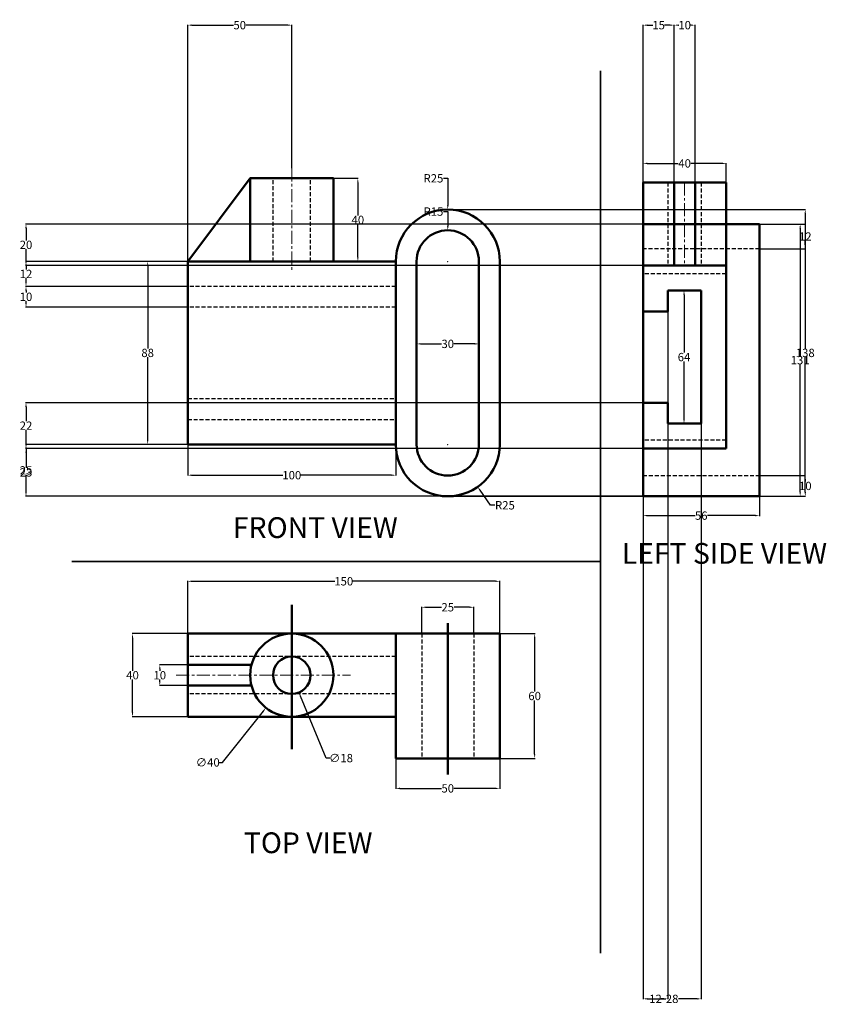
# Model space of a CAD drawing. Units: millimetres. Extents: x -141 to 252, y -566 to 219.
# Tile 1 of 2: x -141 to 247, y -566 to -92. Entities that reach past the tile are written whole.
import ezdxf

# ---------------------------------------------------------------- set-up
doc = ezdxf.new("R2010")
doc.units = ezdxf.units.MM
doc.header["$MEASUREMENT"] = 0
doc.linetypes.add('CENTER', pattern=[2, 1.25, -0.25, 0.25, -0.25])
doc.linetypes.add('HIDDEN', pattern=[9.525, 6.35, -3.175])
for name, color, linetype, lineweight in [('M-CNTR', 1, 'CENTER', 18), ('M-DIMS', 2, 'Continuous', 25), ('M-HIDN', 2, 'HIDDEN', 25), ('M-OUTL', 7, 'Continuous', 50), ('M-TEXT', 7, 'Continuous', 25), ('M-TTLB', 8, 'Continuous', 35)]:
    doc.layers.add(name, color=color, linetype=linetype, lineweight=lineweight)
doc.styles.get("Standard").update_dxf_attribs({"font": 'arial.ttf'})
doc.dimstyles.get("Standard").update_dxf_attribs({"dimtxt": 4, "dimasz": 2, "dimexe": 0.18, "dimexo": 0.0625, "dimgap": 0.09, "dimtad": 0, "dimtih": 1, "dimtoh": 1, "dimdec": 0, "dimzin": 0, "dimdsep": 46, "dimtxsty": 'Standard', "dimcen": 0.09, "dimadec": 0, "dimazin": 0, "dimtfac": 1, "dimtdec": 0, "dimtofl": 0, "dimtmove": 0, "dimatfit": 3, "dimfxl": 1, "dimtolj": 1, "dimtzin": 0, "dimarcsym": 0})

# ---------------------------------------------------------------- blocks, each defined once
blk = doc.blocks.new('*D12')
at = {"layer": 'Defpoints', "color": 0, "transparency": 16777216}
for p in [(-59.91, -208.36), (-79.17, -296.36), (-59.91, -296.36)]:
    blk.add_point(p, dxfattribs=at)
at = {"layer": 'M-DIMS', "color": 0, "lineweight": -2, "transparency": 16777216}
for p, q in [((-59.97, -208.36), (-79.35, -208.36)), ((-79.17, -210.36), (-79.17, -250.22)), ((-79.17, -294.36), (-79.17, -254.49)), ((-59.97, -296.36), (-79.35, -296.36))]:
    blk.add_line(p, q, dxfattribs=at)
at = {"layer": 'M-DIMS', "color": 0, "transparency": 16777216}
for points in [[(-79.5, -210.36), (-78.84, -210.36), (-79.17, -208.36)], [(-79.5, -294.36), (-78.84, -294.36), (-79.17, -296.36)]]:
    blk.add_solid(points, dxfattribs=at)
at = {"layer": 'M-DIMS', "color": 0, "transparency": 16777216, "insert": (-79.17, -252.36), "char_height": 4, "attachment_point": 5}
blk.add_mtext('\\A1;88', dxfattribs=at)
blk = doc.blocks.new('*D13')
at = {"layer": 'Defpoints', "color": 0, "transparency": 16777216}
for p in [(-59.91, -296.36), (40.09, -296.36), (40.09, -311.2)]:
    blk.add_point(p, dxfattribs=at)
at = {"layer": 'M-DIMS', "color": 0, "lineweight": -2, "transparency": 16777216}
for p, q in [((-59.91, -296.42), (-59.91, -311.38)), ((40.09, -296.42), (40.09, -311.38)), ((-57.91, -311.2), (-14.22, -311.2)), ((38.09, -311.2), (-5.59, -311.2))]:
    blk.add_line(p, q, dxfattribs=at)
at = {"layer": 'M-DIMS', "color": 0, "transparency": 16777216}
for points in [[(-57.91, -310.87), (-57.91, -311.54), (-59.91, -311.2)], [(38.09, -310.87), (38.09, -311.54), (40.09, -311.2)]]:
    blk.add_solid(points, dxfattribs=at)
at = {"layer": 'M-DIMS', "color": 0, "transparency": 16777216, "insert": (-9.91, -311.2), "char_height": 4, "attachment_point": 5}
blk.add_mtext('\\A1;100', dxfattribs=at)
blk = doc.blocks.new('*D14')
at = {"layer": 'Defpoints', "color": 0, "transparency": 16777216}
for p in [(10.09, -168.36), (21.87, -168.36), (10.09, -208.36)]:
    blk.add_point(p, dxfattribs=at)
at = {"layer": 'M-DIMS', "color": 0, "lineweight": -2, "transparency": 16777216}
for p, q in [((10.15, -168.36), (22.05, -168.36)), ((21.87, -170.36), (21.87, -186.22)), ((21.87, -206.36), (21.87, -190.49)), ((10.15, -208.36), (22.05, -208.36))]:
    blk.add_line(p, q, dxfattribs=at)
at = {"layer": 'M-DIMS', "color": 0, "transparency": 16777216}
for points in [[(21.54, -170.36), (22.2, -170.36), (21.87, -168.36)], [(21.54, -206.36), (22.2, -206.36), (21.87, -208.36)]]:
    blk.add_solid(points, dxfattribs=at)
at = {"layer": 'M-DIMS', "color": 0, "transparency": 16777216, "insert": (21.87, -188.36), "char_height": 4, "attachment_point": 5}
blk.add_mtext('\\A1;40', dxfattribs=at)
blk = doc.blocks.new('*D15')
at = {"layer": 'Defpoints', "color": 0, "transparency": 16777216}
for p in [(80.09, -248.02), (50.09, -252.36), (80.09, -252.36)]:
    blk.add_point(p, dxfattribs=at)
at = {"layer": 'M-DIMS', "color": 0, "lineweight": -2, "transparency": 16777216}
for p, q in [((50.09, -252.29), (50.09, -247.84)), ((52.09, -248.02), (62.15, -248.02)), ((78.09, -248.02), (68.04, -248.02)), ((80.09, -252.29), (80.09, -247.84))]:
    blk.add_line(p, q, dxfattribs=at)
at = {"layer": 'M-DIMS', "color": 0, "transparency": 16777216}
for points in [[(52.09, -247.69), (52.09, -248.36), (50.09, -248.02)], [(78.09, -247.69), (78.09, -248.36), (80.09, -248.02)]]:
    blk.add_solid(points, dxfattribs=at)
at = {"layer": 'M-DIMS', "color": 0, "transparency": 16777216, "insert": (65.09, -248.02), "char_height": 4, "attachment_point": 5}
blk.add_mtext('\\A1;30', dxfattribs=at)
blk = doc.blocks.new('*D16')
at = {"layer": 'Defpoints', "color": 0, "transparency": 16777216}
for p in [(65.09, -296.36), (79.46, -316.81)]:
    blk.add_point(p, dxfattribs=at)
at = {"layer": 'M-DIMS', "color": 0, "lineweight": -2, "transparency": 16777216}
for p, q in [((65, -296.36), (65.18, -296.36)), ((65.09, -296.45), (65.09, -296.27)), ((85.69, -325.67), (80.61, -318.45)), ((87.69, -325.67), (85.69, -325.67))]:
    blk.add_line(p, q, dxfattribs=at)
at = {"layer": 'M-DIMS', "color": 0, "transparency": 16777216}
blk.add_solid([(80.89, -318.26), (80.34, -318.64), (79.46, -316.81)], dxfattribs=at)
at = {"layer": 'M-DIMS', "color": 0, "transparency": 16777216, "insert": (92.57, -325.67), "char_height": 4, "attachment_point": 5}
blk.add_mtext('\\A1;R25', dxfattribs=at)
blk = doc.blocks.new('*D17')
at = {"layer": 'Defpoints', "color": 0, "transparency": 16777216}
for p in [(-59.91, -387.43), (-86.46, -427.43), (-59.91, -427.43)]:
    blk.add_point(p, dxfattribs=at)
at = {"layer": 'M-DIMS', "color": 0, "lineweight": -2, "transparency": 16777216}
for p, q in [((-59.97, -387.43), (-86.64, -387.43)), ((-86.46, -389.43), (-86.46, -405.3)), ((-86.46, -425.43), (-86.46, -409.56)), ((-59.97, -427.43), (-86.64, -427.43))]:
    blk.add_line(p, q, dxfattribs=at)
at = {"layer": 'M-DIMS', "color": 0, "transparency": 16777216}
for points in [[(-86.8, -389.43), (-86.13, -389.43), (-86.46, -387.43)], [(-86.8, -425.43), (-86.13, -425.43), (-86.46, -427.43)]]:
    blk.add_solid(points, dxfattribs=at)
at = {"layer": 'M-DIMS', "color": 0, "transparency": 16777216, "insert": (-86.46, -407.43), "char_height": 4, "attachment_point": 5}
blk.add_mtext('\\A1;40', dxfattribs=at)
blk = doc.blocks.new('*D18')
at = {"layer": 'Defpoints', "color": 0, "transparency": 16777216}
for p in [(-59.91, -402.43), (-73.35, -412.43), (-59.91, -412.43)]:
    blk.add_point(p, dxfattribs=at)
at = {"layer": 'M-DIMS', "color": 0, "lineweight": -2, "transparency": 16777216}
for p, q in [((-59.97, -402.43), (-73.53, -402.43)), ((-73.35, -404.43), (-73.35, -405.3)), ((-73.35, -410.43), (-73.35, -409.56)), ((-59.97, -412.43), (-73.53, -412.43))]:
    blk.add_line(p, q, dxfattribs=at)
at = {"layer": 'M-DIMS', "color": 0, "transparency": 16777216}
for points in [[(-73.69, -404.43), (-73.02, -404.43), (-73.35, -402.43)], [(-73.69, -410.43), (-73.02, -410.43), (-73.35, -412.43)]]:
    blk.add_solid(points, dxfattribs=at)
at = {"layer": 'M-DIMS', "color": 0, "transparency": 16777216, "insert": (-73.35, -407.43), "char_height": 4, "attachment_point": 5}
blk.add_mtext('\\A1;10', dxfattribs=at)
blk = doc.blocks.new('*D19')
at = {"layer": 'Defpoints', "color": 0, "transparency": 16777216}
for p in [(90.09, -362.24), (-59.91, -387.43), (90.09, -387.43)]:
    blk.add_point(p, dxfattribs=at)
at = {"layer": 'M-DIMS', "color": 0, "lineweight": -2, "transparency": 16777216}
for p, q in [((-59.91, -387.37), (-59.91, -362.06)), ((-57.91, -362.24), (10.78, -362.24)), ((88.09, -362.24), (19.41, -362.24)), ((90.09, -387.37), (90.09, -362.06))]:
    blk.add_line(p, q, dxfattribs=at)
at = {"layer": 'M-DIMS', "color": 0, "transparency": 16777216}
for points in [[(-57.91, -361.9), (-57.91, -362.57), (-59.91, -362.24)], [(88.09, -361.9), (88.09, -362.57), (90.09, -362.24)]]:
    blk.add_solid(points, dxfattribs=at)
at = {"layer": 'M-DIMS', "color": 0, "transparency": 16777216, "insert": (15.09, -362.24), "char_height": 4, "attachment_point": 5}
blk.add_mtext('\\A1;150', dxfattribs=at)
blk = doc.blocks.new('*D20')
at = {"layer": 'Defpoints', "color": 0, "transparency": 16777216}
for p in [(77.59, -374.73), (52.59, -387.43), (77.59, -387.43)]:
    blk.add_point(p, dxfattribs=at)
at = {"layer": 'M-DIMS', "color": 0, "lineweight": -2, "transparency": 16777216}
for p, q in [((52.59, -387.37), (52.59, -374.55)), ((54.59, -374.73), (62.09, -374.73)), ((75.59, -374.73), (68.1, -374.73)), ((77.59, -387.37), (77.59, -374.55))]:
    blk.add_line(p, q, dxfattribs=at)
at = {"layer": 'M-DIMS', "color": 0, "transparency": 16777216}
for points in [[(54.59, -374.4), (54.59, -375.06), (52.59, -374.73)], [(75.59, -374.4), (75.59, -375.06), (77.59, -374.73)]]:
    blk.add_solid(points, dxfattribs=at)
at = {"layer": 'M-DIMS', "color": 0, "transparency": 16777216, "insert": (65.09, -374.73), "char_height": 4, "attachment_point": 5}
blk.add_mtext('\\A1;25', dxfattribs=at)
blk = doc.blocks.new('*D21')
at = {"layer": 'Defpoints', "color": 0, "transparency": 16777216}
for p in [(40.09, -447.43), (90.09, -447.43), (40.09, -461.88)]:
    blk.add_point(p, dxfattribs=at)
at = {"layer": 'M-DIMS', "color": 0, "lineweight": -2, "transparency": 16777216}
for p, q in [((40.09, -447.5), (40.09, -462.06)), ((90.09, -447.5), (90.09, -462.06)), ((42.09, -461.88), (62.14, -461.88)), ((88.09, -461.88), (68.04, -461.88))]:
    blk.add_line(p, q, dxfattribs=at)
at = {"layer": 'M-DIMS', "color": 0, "transparency": 16777216}
for points in [[(42.09, -461.55), (42.09, -462.21), (40.09, -461.88)], [(88.09, -461.55), (88.09, -462.21), (90.09, -461.88)]]:
    blk.add_solid(points, dxfattribs=at)
at = {"layer": 'M-DIMS', "color": 0, "transparency": 16777216, "insert": (65.09, -461.88), "char_height": 4, "attachment_point": 5}
blk.add_mtext('\\A1;50', dxfattribs=at)
blk = doc.blocks.new('*D22')
at = {"layer": 'Defpoints', "color": 0, "transparency": 16777216}
for p in [(90.09, -387.43), (90.09, -447.43), (106.86, -447.43)]:
    blk.add_point(p, dxfattribs=at)
at = {"layer": 'M-DIMS', "color": 0, "lineweight": -2, "transparency": 16777216}
for p, q in [((90.15, -387.43), (107.04, -387.43)), ((106.86, -389.43), (106.86, -415.3)), ((106.86, -445.43), (106.86, -419.56)), ((90.15, -447.43), (107.04, -447.43))]:
    blk.add_line(p, q, dxfattribs=at)
at = {"layer": 'M-DIMS', "color": 0, "transparency": 16777216}
for points in [[(106.53, -389.43), (107.19, -389.43), (106.86, -387.43)], [(106.53, -445.43), (107.19, -445.43), (106.86, -447.43)]]:
    blk.add_solid(points, dxfattribs=at)
at = {"layer": 'M-DIMS', "color": 0, "transparency": 16777216, "insert": (106.86, -417.43), "char_height": 4, "attachment_point": 5}
blk.add_mtext('\\A1;60', dxfattribs=at)
blk = doc.blocks.new('*D23')
at = {"layer": 'Defpoints', "color": 0, "transparency": 16777216}
for p in [(2.52, -391.76), (-22.33, -423.11)]:
    blk.add_point(p, dxfattribs=at)
at = {"layer": 'M-DIMS', "color": 0, "lineweight": -2, "transparency": 16777216}
for p, q in [((-9.91, -407.52), (-9.91, -407.34)), ((-10, -407.43), (-9.82, -407.43)), ((-43.16, -449.39), (-23.57, -424.67)), ((-45.16, -449.39), (-43.16, -449.39))]:
    blk.add_line(p, q, dxfattribs=at)
at = {"layer": 'M-DIMS', "color": 0, "transparency": 16777216}
blk.add_solid([(-23.84, -424.47), (-23.31, -424.88), (-22.33, -423.11)], dxfattribs=at)
at = {"layer": 'M-DIMS', "color": 0, "transparency": 16777216, "insert": (-50.29, -449.39), "char_height": 4, "attachment_point": 5}
blk.add_mtext('\\A1;∅40', dxfattribs=at)
blk = doc.blocks.new('*D24')
at = {"layer": 'Defpoints', "color": 0, "transparency": 16777216}
for p in [(-13.36, -399.12), (-6.46, -415.75)]:
    blk.add_point(p, dxfattribs=at)
at = {"layer": 'M-DIMS', "color": 0, "lineweight": -2, "transparency": 16777216}
for p, q in [((-9.91, -407.52), (-9.91, -407.34)), ((-10, -407.43), (-9.82, -407.43)), ((6.63, -447.3), (-5.69, -417.59)), ((8.63, -447.3), (6.63, -447.3))]:
    blk.add_line(p, q, dxfattribs=at)
at = {"layer": 'M-DIMS', "color": 0, "transparency": 16777216}
blk.add_solid([(-5.39, -417.47), (-6, -417.72), (-6.46, -415.75)], dxfattribs=at)
at = {"layer": 'M-DIMS', "color": 0, "transparency": 16777216, "insert": (13.76, -447.3), "char_height": 4, "attachment_point": 5}
blk.add_mtext('\\A1;∅18', dxfattribs=at)
blk = doc.blocks.new('*D25')
at = {"layer": 'Defpoints', "color": 0, "transparency": 16777216}
for p in [(198.96, -161.18), (158.96, -170.36), (198.96, -170.36)]:
    blk.add_point(p, dxfattribs=at)
at = {"layer": 'M-DIMS', "color": 0, "lineweight": -2, "transparency": 16777216}
for p, q in [((158.96, -170.29), (158.96, -161)), ((198.96, -170.29), (198.96, -161)), ((160.96, -161.18), (175.93, -161.18)), ((196.96, -161.18), (181.99, -161.18))]:
    blk.add_line(p, q, dxfattribs=at)
at = {"layer": 'M-DIMS', "color": 0, "transparency": 16777216}
for points in [[(160.96, -160.84), (160.96, -161.51), (158.96, -161.18)], [(196.96, -160.84), (196.96, -161.51), (198.96, -161.18)]]:
    blk.add_solid(points, dxfattribs=at)
at = {"layer": 'M-DIMS', "color": 0, "transparency": 16777216, "insert": (178.96, -161.18), "char_height": 4, "attachment_point": 5}
blk.add_mtext('\\A1;40', dxfattribs=at)
blk = doc.blocks.new('*D26')
at = {"layer": 'Defpoints', "color": 0, "transparency": 16777216}
for p in [(186.96, -222.36), (178.67, -286.36), (186.96, -286.36)]:
    blk.add_point(p, dxfattribs=at)
at = {"layer": 'M-DIMS', "color": 0, "lineweight": -2, "transparency": 16777216}
for p, q in [((186.9, -222.36), (178.49, -222.36)), ((178.67, -224.36), (178.67, -252.22)), ((178.67, -284.36), (178.67, -256.49)), ((186.9, -286.36), (178.49, -286.36))]:
    blk.add_line(p, q, dxfattribs=at)
at = {"layer": 'M-DIMS', "color": 0, "transparency": 16777216}
for points in [[(178.34, -224.36), (179.01, -224.36), (178.67, -222.36)], [(178.34, -284.36), (179.01, -284.36), (178.67, -286.36)]]:
    blk.add_solid(points, dxfattribs=at)
at = {"layer": 'M-DIMS', "color": 0, "transparency": 16777216, "insert": (178.67, -254.36), "char_height": 4, "attachment_point": 5}
blk.add_mtext('\\A1;64', dxfattribs=at)
blk = doc.blocks.new('*D27')
at = {"layer": 'Defpoints', "color": 0, "transparency": 16777216}
for p in [(214.96, -190.36), (214.96, -321.36), (234.5, -321.36)]:
    blk.add_point(p, dxfattribs=at)
at = {"layer": 'M-DIMS', "color": 0, "lineweight": -2, "transparency": 16777216}
for p, q in [((215.02, -190.36), (234.68, -190.36)), ((234.5, -192.36), (234.5, -253.72)), ((234.5, -319.36), (234.5, -257.99)), ((215.02, -321.36), (234.68, -321.36))]:
    blk.add_line(p, q, dxfattribs=at)
at = {"layer": 'M-DIMS', "color": 0, "transparency": 16777216}
for points in [[(234.17, -192.36), (234.84, -192.36), (234.5, -190.36)], [(234.17, -319.36), (234.84, -319.36), (234.5, -321.36)]]:
    blk.add_solid(points, dxfattribs=at)
at = {"layer": 'M-DIMS', "color": 0, "transparency": 16777216, "insert": (234.5, -255.86), "char_height": 4, "attachment_point": 5}
blk.add_mtext('\\A1;131', dxfattribs=at)
blk = doc.blocks.new('*D28')
at = {"layer": 'Defpoints', "color": 0, "transparency": 16777216}
for p in [(158.96, -321.36), (214.96, -321.36), (214.96, -330.65)]:
    blk.add_point(p, dxfattribs=at)
at = {"layer": 'M-DIMS', "color": 0, "lineweight": -2, "transparency": 16777216}
for p, q in [((158.96, -321.42), (158.96, -330.83)), ((214.96, -321.42), (214.96, -330.83)), ((160.96, -330.65), (184, -330.65)), ((212.96, -330.65), (189.91, -330.65))]:
    blk.add_line(p, q, dxfattribs=at)
at = {"layer": 'M-DIMS', "color": 0, "transparency": 16777216}
for points in [[(160.96, -330.31), (160.96, -330.98), (158.96, -330.65)], [(212.96, -330.31), (212.96, -330.98), (214.96, -330.65)]]:
    blk.add_solid(points, dxfattribs=at)
at = {"layer": 'M-DIMS', "color": 0, "transparency": 16777216, "insert": (186.96, -330.65), "char_height": 4, "attachment_point": 5}
blk.add_mtext('\\A1;56', dxfattribs=at)
blk = doc.blocks.new('*D29')
at = {"layer": 'Defpoints', "color": 0, "transparency": 16777216}
for p in [(-9.91, -94.67), (-9.91, -163.57), (-59.91, -208.36)]:
    blk.add_point(p, dxfattribs=at)
at = {"layer": 'M-DIMS', "color": 0, "lineweight": -2, "transparency": 16777216}
for p, q in [((-59.91, -208.29), (-59.91, -94.49)), ((-57.91, -94.67), (-37.86, -94.67)), ((-11.91, -94.67), (-31.96, -94.67)), ((-9.91, -163.5), (-9.91, -94.49))]:
    blk.add_line(p, q, dxfattribs=at)
at = {"layer": 'M-DIMS', "color": 0, "transparency": 16777216}
for points in [[(-57.91, -94.33), (-57.91, -95), (-59.91, -94.67)], [(-11.91, -94.33), (-11.91, -95), (-9.91, -94.67)]]:
    blk.add_solid(points, dxfattribs=at)
at = {"layer": 'M-DIMS', "color": 0, "transparency": 16777216, "insert": (-34.91, -94.67), "char_height": 4, "attachment_point": 5}
blk.add_mtext('\\A1;50', dxfattribs=at)
blk = doc.blocks.new('*D30')
at = {"layer": 'Defpoints', "color": 0, "transparency": 16777216}
for p in [(-59.91, -296.36), (-137.67, -321.36), (65.09, -321.36)]:
    blk.add_point(p, dxfattribs=at)
at = {"layer": 'M-DIMS', "color": 0, "lineweight": -2, "transparency": 16777216}
for p, q in [((-59.97, -296.36), (-137.85, -296.36)), ((-137.67, -298.36), (-137.67, -306.72)), ((-137.67, -319.36), (-137.67, -310.99)), ((65.03, -321.36), (-137.85, -321.36))]:
    blk.add_line(p, q, dxfattribs=at)
at = {"layer": 'M-DIMS', "color": 0, "transparency": 16777216}
for points in [[(-138, -298.36), (-137.33, -298.36), (-137.67, -296.36)], [(-138, -319.36), (-137.33, -319.36), (-137.67, -321.36)]]:
    blk.add_solid(points, dxfattribs=at)
at = {"layer": 'M-DIMS', "color": 0, "transparency": 16777216, "insert": (-137.67, -308.86), "char_height": 4, "attachment_point": 5}
blk.add_mtext('\\A1;25', dxfattribs=at)
blk = doc.blocks.new('*D31')
at = {"layer": 'Defpoints', "color": 0, "transparency": 16777216}
for p in [(65.09, -183.36), (236.96, -183.36), (65.09, -321.36)]:
    blk.add_point(p, dxfattribs=at)
at = {"layer": 'M-DIMS', "color": 0, "lineweight": -2, "transparency": 16777216}
for p, q in [((65.15, -183.36), (237.14, -183.36)), ((236.96, -185.36), (236.96, -250.22)), ((236.96, -319.36), (236.96, -254.49)), ((65.15, -321.36), (237.14, -321.36))]:
    blk.add_line(p, q, dxfattribs=at)
at = {"layer": 'M-DIMS', "color": 0, "transparency": 16777216}
for points in [[(236.62, -185.36), (237.29, -185.36), (236.96, -183.36)], [(236.62, -319.36), (237.29, -319.36), (236.96, -321.36)]]:
    blk.add_solid(points, dxfattribs=at)
at = {"layer": 'M-DIMS', "color": 0, "transparency": 16777216, "insert": (236.96, -252.36), "char_height": 4, "attachment_point": 5}
blk.add_mtext('\\A1;138', dxfattribs=at)
blk = doc.blocks.new('*D32')
at = {"layer": 'Defpoints', "color": 0, "transparency": 16777216}
for p in [(158.96, -190.36), (-137.67, -210.36), (158.96, -210.36)]:
    blk.add_point(p, dxfattribs=at)
at = {"layer": 'M-DIMS', "color": 0, "lineweight": -2, "transparency": 16777216}
for p, q in [((158.9, -190.36), (-137.85, -190.36)), ((-137.67, -192.36), (-137.67, -198.22)), ((-137.67, -208.36), (-137.67, -202.49)), ((158.9, -210.36), (-137.85, -210.36))]:
    blk.add_line(p, q, dxfattribs=at)
at = {"layer": 'M-DIMS', "color": 0, "transparency": 16777216}
for points in [[(-138, -192.36), (-137.33, -192.36), (-137.67, -190.36)], [(-138, -208.36), (-137.33, -208.36), (-137.67, -210.36)]]:
    blk.add_solid(points, dxfattribs=at)
at = {"layer": 'M-DIMS', "color": 0, "transparency": 16777216, "insert": (-137.67, -200.36), "char_height": 4, "attachment_point": 5}
blk.add_mtext('\\A1;20', dxfattribs=at)
blk = doc.blocks.new('*D33')
at = {"layer": 'Defpoints', "color": 0, "transparency": 16777216}
for p in [(-59.91, -208.36), (-137.67, -220.36), (-59.91, -220.36)]:
    blk.add_point(p, dxfattribs=at)
at = {"layer": 'M-DIMS', "color": 0, "lineweight": -2, "transparency": 16777216}
for p, q in [((-59.97, -208.36), (-137.85, -208.36)), ((-137.67, -210.36), (-137.67, -212.26)), ((-137.67, -218.36), (-137.67, -216.46)), ((-59.97, -220.36), (-137.85, -220.36))]:
    blk.add_line(p, q, dxfattribs=at)
at = {"layer": 'M-DIMS', "color": 0, "transparency": 16777216}
for points in [[(-138, -210.36), (-137.33, -210.36), (-137.67, -208.36)], [(-138, -218.36), (-137.33, -218.36), (-137.67, -220.36)]]:
    blk.add_solid(points, dxfattribs=at)
at = {"layer": 'M-DIMS', "color": 0, "transparency": 16777216, "insert": (-137.67, -214.36), "char_height": 4, "attachment_point": 5}
blk.add_mtext('\\A1;12', dxfattribs=at)
blk = doc.blocks.new('*D34')
at = {"layer": 'Defpoints', "color": 0, "transparency": 16777216}
for p in [(-59.91, -220.36), (-137.67, -230.36), (-59.91, -230.36)]:
    blk.add_point(p, dxfattribs=at)
at = {"layer": 'M-DIMS', "color": 0, "lineweight": -2, "transparency": 16777216}
for p, q in [((-59.97, -220.36), (-137.85, -220.36)), ((-137.67, -222.36), (-137.67, -223.22)), ((-59.97, -230.36), (-137.85, -230.36)), ((-137.67, -228.36), (-137.67, -227.49))]:
    blk.add_line(p, q, dxfattribs=at)
at = {"layer": 'M-DIMS', "color": 0, "transparency": 16777216}
for points in [[(-138, -222.36), (-137.33, -222.36), (-137.67, -220.36)], [(-138, -228.36), (-137.33, -228.36), (-137.67, -230.36)]]:
    blk.add_solid(points, dxfattribs=at)
at = {"layer": 'M-DIMS', "color": 0, "transparency": 16777216, "insert": (-137.67, -225.36), "char_height": 4, "attachment_point": 5}
blk.add_mtext('\\A1;10', dxfattribs=at)
blk = doc.blocks.new('*D35')
at = {"layer": 'Defpoints', "color": 0, "transparency": 16777216}
for p in [(158.96, -276.36), (-137.67, -298.36), (158.96, -298.36)]:
    blk.add_point(p, dxfattribs=at)
at = {"layer": 'M-DIMS', "color": 0, "lineweight": -2, "transparency": 16777216}
for p, q in [((158.9, -276.36), (-137.85, -276.36)), ((-137.67, -278.36), (-137.67, -285.26)), ((-137.67, -296.36), (-137.67, -289.46)), ((158.9, -298.36), (-137.85, -298.36))]:
    blk.add_line(p, q, dxfattribs=at)
at = {"layer": 'M-DIMS', "color": 0, "transparency": 16777216}
for points in [[(-138, -278.36), (-137.33, -278.36), (-137.67, -276.36)], [(-138, -296.36), (-137.33, -296.36), (-137.67, -298.36)]]:
    blk.add_solid(points, dxfattribs=at)
at = {"layer": 'M-DIMS', "color": 0, "transparency": 16777216, "insert": (-137.67, -287.36), "char_height": 4, "attachment_point": 5}
blk.add_mtext('\\A1;22', dxfattribs=at)
blk = doc.blocks.new('*D36')
at = {"layer": 'Defpoints', "color": 0, "transparency": 16777216}
for p in [(158.96, -298.36), (-137.67, -321.36), (158.96, -321.36)]:
    blk.add_point(p, dxfattribs=at)
at = {"layer": 'M-DIMS', "color": 0, "lineweight": -2, "transparency": 16777216}
for p, q in [((158.9, -298.36), (-137.85, -298.36)), ((-137.67, -300.36), (-137.67, -307.72)), ((-137.67, -319.36), (-137.67, -311.99)), ((158.9, -321.36), (-137.85, -321.36))]:
    blk.add_line(p, q, dxfattribs=at)
at = {"layer": 'M-DIMS', "color": 0, "transparency": 16777216}
for points in [[(-138, -300.36), (-137.33, -300.36), (-137.67, -298.36)], [(-138, -319.36), (-137.33, -319.36), (-137.67, -321.36)]]:
    blk.add_solid(points, dxfattribs=at)
at = {"layer": 'M-DIMS', "color": 0, "transparency": 16777216, "insert": (-137.67, -309.86), "char_height": 4, "attachment_point": 5}
blk.add_mtext('\\A1;23', dxfattribs=at)
blk = doc.blocks.new('*D37')
at = {"layer": 'Defpoints', "color": 0, "transparency": 16777216}
for p in [(214.96, -190.36), (214.96, -202.36), (236.96, -202.36)]:
    blk.add_point(p, dxfattribs=at)
at = {"layer": 'M-DIMS', "color": 0, "lineweight": -2, "transparency": 16777216}
for p, q in [((215.02, -190.36), (237.14, -190.36)), ((236.96, -192.36), (236.96, -194.26)), ((236.96, -200.36), (236.96, -198.46)), ((215.02, -202.36), (237.14, -202.36))]:
    blk.add_line(p, q, dxfattribs=at)
at = {"layer": 'M-DIMS', "color": 0, "transparency": 16777216}
for points in [[(236.62, -192.36), (237.29, -192.36), (236.96, -190.36)], [(236.62, -200.36), (237.29, -200.36), (236.96, -202.36)]]:
    blk.add_solid(points, dxfattribs=at)
at = {"layer": 'M-DIMS', "color": 0, "transparency": 16777216, "insert": (236.96, -196.36), "char_height": 4, "attachment_point": 5}
blk.add_mtext('\\A1;12', dxfattribs=at)
blk = doc.blocks.new('*D38')
at = {"layer": 'Defpoints', "color": 0, "transparency": 16777216}
for p in [(214.96, -311.36), (236.96, -311.36), (214.96, -321.36)]:
    blk.add_point(p, dxfattribs=at)
at = {"layer": 'M-DIMS', "color": 0, "lineweight": -2, "transparency": 16777216}
for p, q in [((215.02, -311.36), (237.14, -311.36)), ((236.96, -313.36), (236.96, -314.22)), ((215.02, -321.36), (237.14, -321.36)), ((236.96, -319.36), (236.96, -318.49))]:
    blk.add_line(p, q, dxfattribs=at)
at = {"layer": 'M-DIMS', "color": 0, "transparency": 16777216}
for points in [[(236.62, -313.36), (237.29, -313.36), (236.96, -311.36)], [(236.62, -319.36), (237.29, -319.36), (236.96, -321.36)]]:
    blk.add_solid(points, dxfattribs=at)
at = {"layer": 'M-DIMS', "color": 0, "transparency": 16777216, "insert": (236.96, -316.36), "char_height": 4, "attachment_point": 5}
blk.add_mtext('\\A1;10', dxfattribs=at)
blk = doc.blocks.new('*D39')
at = {"layer": 'Defpoints', "color": 0, "transparency": 16777216}
for p in [(158.96, -232.36), (170.96, -232.36), (170.96, -563.14)]:
    blk.add_point(p, dxfattribs=at)
at = {"layer": 'M-DIMS', "color": 0, "lineweight": -2, "transparency": 16777216}
for p, q in [((158.96, -232.42), (158.96, -563.32)), ((170.96, -232.42), (170.96, -563.32)), ((160.96, -563.14), (162.21, -563.14)), ((168.96, -563.14), (167.7, -563.14))]:
    blk.add_line(p, q, dxfattribs=at)
at = {"layer": 'M-DIMS', "color": 0, "transparency": 16777216}
for points in [[(160.96, -562.81), (160.96, -563.48), (158.96, -563.14)], [(168.96, -562.81), (168.96, -563.48), (170.96, -563.14)]]:
    blk.add_solid(points, dxfattribs=at)
at = {"layer": 'M-DIMS', "color": 0, "transparency": 16777216, "insert": (164.96, -563.14), "char_height": 4, "attachment_point": 5}
blk.add_mtext('\\A1;12', dxfattribs=at)
blk = doc.blocks.new('*D40')
at = {"layer": 'Defpoints', "color": 0, "transparency": 16777216}
for p in [(158.96, -214.36), (186.96, -222.36), (186.96, -563.14)]:
    blk.add_point(p, dxfattribs=at)
at = {"layer": 'M-DIMS', "color": 0, "lineweight": -2, "transparency": 16777216}
for p, q in [((158.96, -214.42), (158.96, -563.32)), ((186.96, -222.42), (186.96, -563.32)), ((160.96, -563.14), (169.96, -563.14)), ((184.96, -563.14), (175.95, -563.14))]:
    blk.add_line(p, q, dxfattribs=at)
at = {"layer": 'M-DIMS', "color": 0, "transparency": 16777216}
for points in [[(160.96, -562.81), (160.96, -563.48), (158.96, -563.14)], [(184.96, -562.81), (184.96, -563.48), (186.96, -563.14)]]:
    blk.add_solid(points, dxfattribs=at)
at = {"layer": 'M-DIMS', "color": 0, "transparency": 16777216, "insert": (172.96, -563.14), "char_height": 4, "attachment_point": 5}
blk.add_mtext('\\A1;28', dxfattribs=at)
blk = doc.blocks.new('*D41')
at = {"layer": 'Defpoints', "color": 0, "transparency": 16777216}
for p in [(173.96, -94.67), (158.96, -170.36), (173.96, -170.36)]:
    blk.add_point(p, dxfattribs=at)
at = {"layer": 'M-DIMS', "color": 0, "lineweight": -2, "transparency": 16777216}
for p, q in [((158.96, -170.29), (158.96, -94.49)), ((160.96, -94.67), (163.68, -94.67)), ((171.96, -94.67), (169.24, -94.67)), ((173.96, -170.29), (173.96, -94.49))]:
    blk.add_line(p, q, dxfattribs=at)
at = {"layer": 'M-DIMS', "color": 0, "transparency": 16777216}
for points in [[(160.96, -94.33), (160.96, -95), (158.96, -94.67)], [(171.96, -94.33), (171.96, -95), (173.96, -94.67)]]:
    blk.add_solid(points, dxfattribs=at)
at = {"layer": 'M-DIMS', "color": 0, "transparency": 16777216, "insert": (166.46, -94.67), "char_height": 4, "attachment_point": 5}
blk.add_mtext('\\A1;15', dxfattribs=at)
blk = doc.blocks.new('*D42')
at = {"layer": 'Defpoints', "color": 0, "transparency": 16777216}
for p in [(183.96, -94.67), (173.96, -170.36), (183.96, -170.36)]:
    blk.add_point(p, dxfattribs=at)
at = {"layer": 'M-DIMS', "color": 0, "lineweight": -2, "transparency": 16777216}
for p, q in [((173.96, -170.29), (173.96, -94.49)), ((175.96, -94.67), (176.2, -94.67)), ((181.96, -94.67), (181.72, -94.67)), ((183.96, -170.29), (183.96, -94.49))]:
    blk.add_line(p, q, dxfattribs=at)
at = {"layer": 'M-DIMS', "color": 0, "transparency": 16777216}
for points in [[(175.96, -94.33), (175.96, -95), (173.96, -94.67)], [(181.96, -94.33), (181.96, -95), (183.96, -94.67)]]:
    blk.add_solid(points, dxfattribs=at)
at = {"layer": 'M-DIMS', "color": 0, "transparency": 16777216, "insert": (178.96, -94.67), "char_height": 4, "attachment_point": 5}
blk.add_mtext('\\A1;10', dxfattribs=at)
blk = doc.blocks.new('*D43')
at = {"layer": 'Defpoints', "color": 0, "transparency": 16777216}
for p in [(65.09, -183.36), (65.09, -208.36)]:
    blk.add_point(p, dxfattribs=at)
at = {"layer": 'M-DIMS', "color": 0, "lineweight": -2, "transparency": 16777216}
for p, q in [((63.09, -168.36), (65.09, -168.36)), ((65.09, -168.36), (65.09, -181.36)), ((65, -208.36), (65.18, -208.36)), ((65.09, -208.45), (65.09, -208.27))]:
    blk.add_line(p, q, dxfattribs=at)
at = {"layer": 'M-DIMS', "color": 0, "transparency": 16777216}
blk.add_solid([(65.43, -181.36), (64.76, -181.36), (65.09, -183.36)], dxfattribs=at)
at = {"layer": 'M-DIMS', "color": 0, "transparency": 16777216, "insert": (58.21, -168.36), "char_height": 4, "attachment_point": 5}
blk.add_mtext('\\A1;R25', dxfattribs=at)
blk = doc.blocks.new('*D44')
at = {"layer": 'Defpoints', "color": 0, "transparency": 16777216}
for p in [(65.09, -193.36), (65.09, -208.36)]:
    blk.add_point(p, dxfattribs=at)
at = {"layer": 'M-DIMS', "color": 0, "lineweight": -2, "transparency": 16777216}
for p, q in [((63.09, -184.36), (65.09, -184.36)), ((65.09, -184.36), (65.09, -191.36)), ((65, -208.36), (65.18, -208.36)), ((65.09, -208.45), (65.09, -208.27))]:
    blk.add_line(p, q, dxfattribs=at)
at = {"layer": 'M-DIMS', "color": 0, "transparency": 16777216}
blk.add_solid([(65.43, -191.36), (64.76, -191.36), (65.09, -193.36)], dxfattribs=at)
at = {"layer": 'M-DIMS', "color": 0, "transparency": 16777216, "insert": (58.21, -184.36), "char_height": 4, "attachment_point": 5}
blk.add_mtext('\\A1;R15', dxfattribs=at)

msp = doc.modelspace()

# ---------------------------------------------------------------- linework, layer by layer
at = {"layer": 'M-CNTR', "ltscale": 5}
for p, q in [((-9.91, -163.57), (-9.91, -213.21)), ((178.96, -170.36), (178.96, -210.36)), ((65.09, -382.4), (65.09, -455.15)), ((-65.47, -407.43), (18.39, -407.43))]:
    msp.add_line(p, q, dxfattribs=at)
at = {"layer": 'M-HIDN', "ltscale": 0.3}
for p, q in [((-18.91, -208.36), (-18.91, -168.36)), ((-0.91, -208.36), (-0.91, -168.36)), ((170.96, -170.36), (170.96, -210.36)), ((186.96, -170.36), (186.96, -210.36)), ((198.96, -190.36), (158.96, -190.36)), ((214.96, -202.36), (158.96, -202.36)), ((198.96, -214.36), (158.96, -214.36)), ((40.09, -220.36), (-59.91, -220.36)), ((40.09, -230.36), (-59.91, -230.36)), ((-59.91, -274.36), (40.09, -274.36)), ((-59.91, -284.36), (40.09, -284.36)), ((198.96, -294.36), (158.96, -294.36)), ((158.96, -311.36), (214.96, -311.36)), ((52.59, -387.43), (52.59, -447.43)), ((77.59, -387.43), (77.59, -447.43)), ((40.09, -398.43), (-59.91, -398.43)), ((40.09, -416.43), (-59.91, -416.43))]:
    msp.add_line(p, q, dxfattribs=at)
at = {"layer": 'M-OUTL'}
for p, q in [((-29.91, -168.36), (-59.91, -208.36)), ((-29.91, -208.36), (-29.91, -168.36)), ((-29.91, -168.36), (10.09, -168.36)), ((10.09, -208.36), (10.09, -168.36)), ((158.96, -170.36), (198.96, -170.36)), ((158.96, -210.36), (158.96, -170.36)), ((173.96, -170.36), (173.96, -210.36)), ((183.96, -170.36), (183.96, -210.36)), ((198.96, -170.36), (198.96, -210.36)), ((198.96, -190.36), (158.96, -190.36)), ((198.96, -190.36), (214.96, -190.36)), ((214.96, -190.36), (214.96, -321.36)), ((-59.91, -208.36), (-59.91, -296.36)), ((40.09, -208.36), (-59.91, -208.36)), ((40.09, -208.36), (-59.91, -208.36)), ((40.09, -296.36), (40.09, -208.36)), ((50.09, -208.36), (50.09, -296.36)), ((80.09, -208.36), (80.09, -296.36)), ((90.09, -208.36), (90.09, -296.36)), ((198.96, -210.36), (158.96, -210.36)), ((158.96, -210.36), (158.96, -232.36)), ((198.96, -298.36), (198.96, -210.36)), ((198.96, -254.36), (198.96, -214.36)), ((170.96, -232.36), (170.96, -222.36)), ((170.96, -222.36), (186.96, -222.36)), ((186.96, -222.36), (186.96, -286.36)), ((158.96, -232.36), (170.96, -232.36)), ((158.96, -232.36), (158.96, -276.36)), ((198.96, -254.36), (198.96, -294.36)), ((170.96, -276.36), (158.96, -276.36)), ((158.96, -276.36), (158.96, -298.36)), ((170.96, -286.36), (170.96, -276.36)), ((186.96, -286.36), (170.96, -286.36)), ((-59.91, -296.36), (40.09, -296.36)), ((158.96, -298.36), (198.96, -298.36)), ((158.96, -321.36), (158.96, -298.36)), ((158.96, -321.36), (214.96, -321.36)), ((138.59, -352.75), (138.59, -352.75)), ((-9.91, -373.6), (-9.91, -443.09)), ((65.09, -382.4), (65.09, -455.15)), ((-59.91, -387.43), (-59.91, -427.43)), ((40.09, -387.43), (-59.91, -387.43)), ((40.09, -427.43), (40.09, -387.43)), ((40.09, -387.43), (90.09, -387.43)), ((90.09, -387.43), (90.09, -447.43)), ((-29.27, -402.43), (-59.91, -402.43)), ((-29.27, -412.43), (-59.91, -412.43)), ((-59.91, -427.43), (40.09, -427.43)), ((40.09, -447.43), (40.09, -427.43)), ((40.09, -427.43), (40.09, -427.43)), ((90.09, -447.43), (40.09, -447.43))]:
    msp.add_line(p, q, dxfattribs=at)
for radius in [20, 9]:
    msp.add_circle((-9.91, -407.43), radius, dxfattribs=at)
for centre, radius, start, end in [((65.09, -208.36), 25, 0, 180), ((65.09, -208.36), 15, 0, 180), ((65.09, -296.36), 25, 180, 0), ((65.09, -296.36), 15, 180, 0)]:
    msp.add_arc(centre, radius, start, end, dxfattribs=at)
at = {"layer": 'M-TTLB'}
for p, q in [((138.59, -352.75), (138.59, -116.67)), ((-115.67, -352.75), (138.59, -352.75)), ((138.59, -352.75), (138.59, -541.14))]:
    msp.add_line(p, q, dxfattribs=at)

# ---------------------------------------------------------------- texts
at = {"layer": 'M-TEXT'}
for s, p in [('FRONT VIEW', (-38.2, -341.42)), ('LEFT SIDE VIEW', (148.77, -353.81)), ('TOP VIEW', (-32.93, -493.05))]:
    msp.add_text(s, height=10, dxfattribs=at).set_placement(p)

# ---------------------------------------------------------------- dimensions: what is measured, and where the dimension line sits
at = {"layer": 'M-DIMS'}
for base, p1, p2, override, picture, middle in [((-9.91, -94.67), (-59.91, -208.36), (-9.91, -163.57), {"dimdec": 0, "dimlfac": 1, "dimrnd": 0, "dimzin": 0, "dimdsep": 46, "dimlunit": 2}, '*D29', (-34.91, -94.67)), ((173.96, -94.67), (158.96, -170.36), (173.96, -170.36), {"dimdec": 0, "dimlfac": 1, "dimrnd": 0, "dimzin": 0, "dimdsep": 46, "dimlunit": 2}, '*D41', (166.46, -94.67)), ((183.96, -94.67), (173.96, -170.36), (183.96, -170.36), {"dimdec": 0, "dimlfac": 1, "dimrnd": 0, "dimzin": 0, "dimdsep": 46, "dimlunit": 2}, '*D42', (178.96, -94.67)), ((198.96, -161.18), (158.96, -170.36), (198.96, -170.36), {"dimclrd": 0, "dimclre": 0, "dimclrt": 0}, '*D25', (178.96, -161.18)), ((186.96, -563.14), (158.96, -214.36), (186.96, -222.36), {"dimdec": 0, "dimlfac": 1, "dimrnd": 0, "dimzin": 0, "dimdsep": 46, "dimlunit": 2}, '*D40', (172.96, -563.14)), ((170.96, -563.14), (158.96, -232.36), (170.96, -232.36), {"dimdec": 0, "dimlfac": 1, "dimrnd": 0, "dimzin": 0, "dimdsep": 46, "dimlunit": 2}, '*D39', (164.96, -563.14)), ((80.09, -248.02), (50.09, -252.36), (80.09, -252.36), {"dimclrd": 0, "dimclre": 0, "dimclrt": 0}, '*D15', (65.09, -248.02)), ((40.09, -311.2), (-59.91, -296.36), (40.09, -296.36), {"dimclrd": 0, "dimclre": 0, "dimclrt": 0}, '*D13', (-9.91, -311.2)), ((214.96, -330.65), (158.96, -321.36), (214.96, -321.36), {"dimclrd": 0, "dimclre": 0, "dimclrt": 0}, '*D28', (186.96, -330.65)), ((90.09, -362.24), (-59.91, -387.43), (90.09, -387.43), {"dimclrd": 0, "dimclre": 0, "dimclrt": 0}, '*D19', (15.09, -362.24)), ((77.59, -374.73), (52.59, -387.43), (77.59, -387.43), {"dimclrd": 0, "dimclre": 0, "dimclrt": 0}, '*D20', (65.09, -374.73)), ((40.09, -461.88), (90.09, -447.43), (40.09, -447.43), {"dimclrd": 0, "dimclre": 0, "dimclrt": 0}, '*D21', (65.09, -461.88))]:
    dim = msp.add_linear_dim(base=base, p1=p1, p2=p2, dimstyle='Standard', override=override, dxfattribs=at)
    dim.commit()
    dim.dimension.update_dxf_attribs({"geometry": picture, "text_midpoint": middle})
for center, mpoint, override, picture, middle in [((65.09, -208.36), (65.09, -183.36), {"dimdec": 0, "dimlfac": 1, "dimrnd": 0, "dimzin": 0, "dimdsep": 46, "dimlunit": 2}, '*D43', (58.21, -168.36)), ((65.09, -208.36), (65.09, -193.36), {"dimdec": 0, "dimlfac": 1, "dimrnd": 0, "dimzin": 0, "dimdsep": 46, "dimlunit": 2}, '*D44', (58.21, -184.36)), ((65.09, -296.36), (79.46, -316.81), {"dimclrd": 0, "dimclre": 0, "dimclrt": 0}, '*D16', (92.57, -325.67))]:
    dim = msp.add_radius_dim(center=center, mpoint=mpoint, dimstyle='Standard', override=override, dxfattribs=at)
    dim.commit()
    dim.dimension.update_dxf_attribs({"geometry": picture, "text_midpoint": middle, "dimtype": 164})
for base, p1, p2, override, picture, middle in [((21.87, -168.36), (10.09, -208.36), (10.09, -168.36), {"dimclrd": 0, "dimclre": 0, "dimclrt": 0}, '*D14', (21.87, -188.36)), ((236.96, -183.36), (65.09, -321.36), (65.09, -183.36), {"dimdec": 0, "dimlfac": 1, "dimrnd": 0, "dimzin": 0, "dimdsep": 46, "dimlunit": 2}, '*D31', (236.96, -252.36)), ((-137.67, -210.36), (158.96, -190.36), (158.96, -210.36), {"dimdec": 0, "dimlfac": 1, "dimrnd": 0, "dimzin": 0, "dimdsep": 46, "dimlunit": 2}, '*D32', (-137.67, -200.36)), ((234.5, -321.36), (214.96, -190.36), (214.96, -321.36), {"dimclrd": 0, "dimclre": 0, "dimclrt": 0}, '*D27', (234.5, -255.86)), ((236.96, -202.36), (214.96, -190.36), (214.96, -202.36), {"dimdec": 0, "dimlfac": 1, "dimrnd": 0, "dimzin": 0, "dimdsep": 46, "dimlunit": 2}, '*D37', (236.96, -196.36)), ((-137.67, -220.36), (-59.91, -208.36), (-59.91, -220.36), {"dimdec": 0, "dimlfac": 1, "dimrnd": 0, "dimzin": 0, "dimdsep": 46, "dimlunit": 2}, '*D33', (-137.67, -214.36)), ((-79.17, -296.36), (-59.91, -208.36), (-59.91, -296.36), {"dimclrd": 0, "dimclre": 0, "dimclrt": 0}, '*D12', (-79.17, -252.36)), ((-137.67, -230.36), (-59.91, -220.36), (-59.91, -230.36), {"dimdec": 0, "dimlfac": 1, "dimrnd": 0, "dimzin": 0, "dimdsep": 46, "dimlunit": 2}, '*D34', (-137.67, -225.36)), ((178.67, -286.36), (186.96, -222.36), (186.96, -286.36), {"dimclrd": 0, "dimclre": 0, "dimclrt": 0}, '*D26', (178.67, -254.36)), ((-137.67, -298.36), (158.96, -276.36), (158.96, -298.36), {"dimdec": 0, "dimlfac": 1, "dimrnd": 0, "dimzin": 0, "dimdsep": 46, "dimlunit": 2}, '*D35', (-137.67, -287.36)), ((-137.67, -321.36), (-59.91, -296.36), (65.09, -321.36), {"dimdec": 0, "dimlfac": 1, "dimrnd": 0, "dimzin": 0, "dimdsep": 46, "dimlunit": 2}, '*D30', (-137.67, -308.86)), ((-137.67, -321.36), (158.96, -298.36), (158.96, -321.36), {"dimdec": 0, "dimlfac": 1, "dimrnd": 0, "dimzin": 0, "dimdsep": 46, "dimlunit": 2}, '*D36', (-137.67, -309.86)), ((236.96, -311.36), (214.96, -321.36), (214.96, -311.36), {"dimdec": 0, "dimlfac": 1, "dimrnd": 0, "dimzin": 0, "dimdsep": 46, "dimlunit": 2}, '*D38', (236.96, -316.36)), ((-86.46, -427.43), (-59.91, -387.43), (-59.91, -427.43), {"dimclrd": 0, "dimclre": 0, "dimclrt": 0}, '*D17', (-86.46, -407.43)), ((106.86, -447.43), (90.09, -387.43), (90.09, -447.43), {"dimclrd": 0, "dimclre": 0, "dimclrt": 0}, '*D22', (106.86, -417.43)), ((-73.35, -412.43), (-59.91, -402.43), (-59.91, -412.43), {"dimclrd": 0, "dimclre": 0, "dimclrt": 0}, '*D18', (-73.35, -407.43))]:
    dim = msp.add_linear_dim(base=base, p1=p1, p2=p2, angle=90, dimstyle='Standard', override=override, dxfattribs=at)
    dim.commit()
    dim.dimension.update_dxf_attribs({"geometry": picture, "text_midpoint": middle})
for p1, p2, picture, middle in [((2.52, -391.76), (-22.33, -423.11), '*D23', (-50.29, -449.39)), ((-13.36, -399.12), (-6.46, -415.75), '*D24', (13.76, -447.3))]:
    dim = msp.add_diameter_dim_2p(p1=p1, p2=p2, dimstyle='Standard', override={"dimclrd": 0, "dimclre": 0, "dimclrt": 0}, dxfattribs=at)
    dim.commit()
    dim.dimension.update_dxf_attribs({"geometry": picture, "text_midpoint": middle, "dimtype": 163})

doc.saveas('drawing.dxf')
